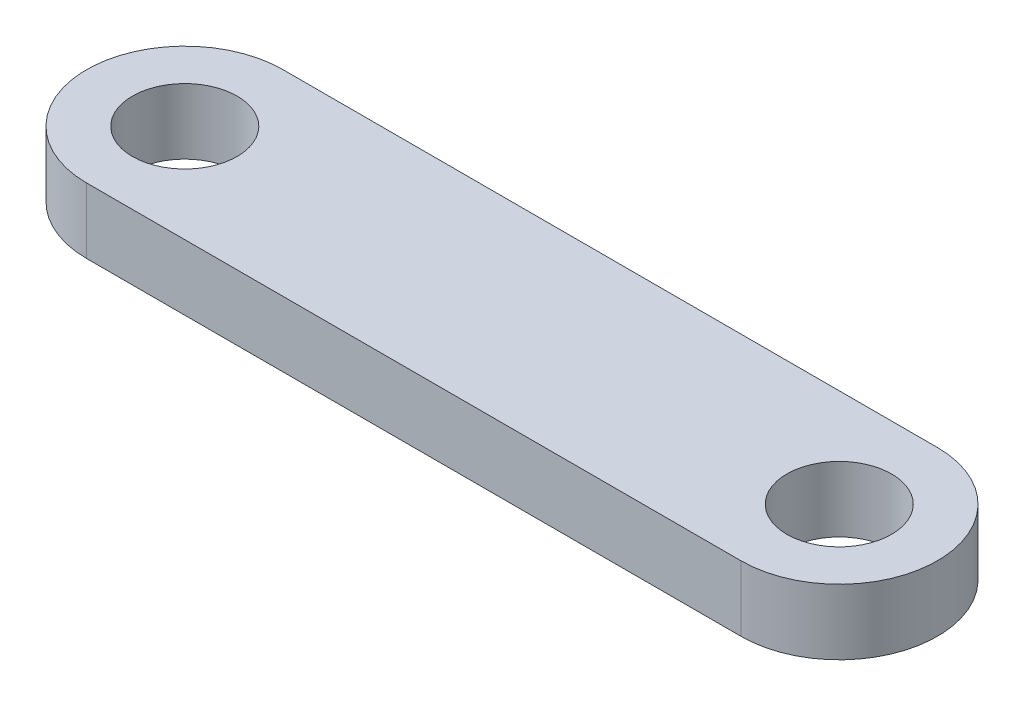
ISO-10303-21;
HEADER;
FILE_DESCRIPTION(('STEP AP214'),'2;1');
FILE_NAME('part.step','',(''),(''),'','','');
FILE_SCHEMA(('AUTOMOTIVE_DESIGN { 1 0 10303 214 1 1 1 1 }'));
ENDSEC;
DATA;
#1=APPLICATION_CONTEXT('core data for automotive mechanical design processes');
#2=APPLICATION_PROTOCOL_DEFINITION('international standard','automotive_design',2000,#1);
#3=PRODUCT_CONTEXT('',#1,'mechanical');
#4=PRODUCT('Part','Part','',(#3));
#5=PRODUCT_RELATED_PRODUCT_CATEGORY('part','',(#4));
#6=PRODUCT_DEFINITION_FORMATION('','',#4);
#7=PRODUCT_DEFINITION_CONTEXT('part definition',#1,'design');
#8=PRODUCT_DEFINITION('design','',#6,#7);
#9=PRODUCT_DEFINITION_SHAPE('','',#8);
#10=(LENGTH_UNIT() NAMED_UNIT(*) SI_UNIT(.MILLI.,.METRE.));
#11=(NAMED_UNIT(*) PLANE_ANGLE_UNIT() SI_UNIT($,.RADIAN.));
#12=(NAMED_UNIT(*) SI_UNIT($,.STERADIAN.) SOLID_ANGLE_UNIT());
#13=UNCERTAINTY_MEASURE_WITH_UNIT(LENGTH_MEASURE(1.E-05),#10,'distance_accuracy_value','');
#14=(GEOMETRIC_REPRESENTATION_CONTEXT(3) GLOBAL_UNCERTAINTY_ASSIGNED_CONTEXT((#13)) GLOBAL_UNIT_ASSIGNED_CONTEXT((#10,
#11,#12)) REPRESENTATION_CONTEXT('',''));
#15=CARTESIAN_POINT('',(0.,0.,0.));
#16=DIRECTION('',(0.,0.,1.));
#17=DIRECTION('',(1.,0.,0.));
#18=AXIS2_PLACEMENT_3D('',#15,#16,#17);
#19=CARTESIAN_POINT('',(-25.,2.5,0.));
#20=DIRECTION('',(0.,-1.,0.));
#21=DIRECTION('',(0.,0.,-1.));
#22=AXIS2_PLACEMENT_3D('',#19,#20,#21);
#23=CYLINDRICAL_SURFACE('',#22,7.5);
#24=CARTESIAN_POINT('',(-25.,-2.5,0.));
#25=DIRECTION('',(0.,1.,0.));
#26=DIRECTION('',(0.,0.,1.));
#27=AXIS2_PLACEMENT_3D('',#24,#25,#26);
#28=CIRCLE('',#27,7.5);
#29=CARTESIAN_POINT('',(-25.,-2.5,-7.5));
#30=VERTEX_POINT('',#29);
#31=CARTESIAN_POINT('',(-25.,-2.5,7.5));
#32=VERTEX_POINT('',#31);
#33=EDGE_CURVE('E102',#30,#32,#28,.T.);
#34=ORIENTED_EDGE('',*,*,#33,.T.);
#35=DIRECTION('',(0.,-1.,0.));
#36=VECTOR('',#35,1.);
#37=CARTESIAN_POINT('',(-25.,2.5,7.5));
#38=LINE('',#37,#36);
#39=CARTESIAN_POINT('',(-25.,2.5,7.5));
#40=VERTEX_POINT('',#39);
#41=EDGE_CURVE('E11',#40,#32,#38,.T.);
#42=ORIENTED_EDGE('',*,*,#41,.F.);
#43=CARTESIAN_POINT('',(-25.,2.5,0.));
#44=DIRECTION('',(0.,1.,0.));
#45=DIRECTION('',(0.,0.,1.));
#46=AXIS2_PLACEMENT_3D('',#43,#44,#45);
#47=CIRCLE('',#46,7.5);
#48=CARTESIAN_POINT('',(-25.,2.5,-7.5));
#49=VERTEX_POINT('',#48);
#50=EDGE_CURVE('E95',#49,#40,#47,.T.);
#51=ORIENTED_EDGE('',*,*,#50,.F.);
#52=DIRECTION('',(0.,-1.,0.));
#53=VECTOR('',#52,1.);
#54=CARTESIAN_POINT('',(-25.,2.5,-7.5));
#55=LINE('',#54,#53);
#56=EDGE_CURVE('E99',#49,#30,#55,.T.);
#57=ORIENTED_EDGE('',*,*,#56,.T.);
#58=EDGE_LOOP('',(#34,#42,#51,#57));
#59=FACE_BOUND('',#58,.T.);
#60=ADVANCED_FACE('F41',(#59),#23,.T.);
#61=CARTESIAN_POINT('',(-25.,2.5,7.5));
#62=DIRECTION('',(0.,0.,-1.));
#63=DIRECTION('',(-1.,0.,0.));
#64=AXIS2_PLACEMENT_3D('',#61,#62,#63);
#65=PLANE('',#64);
#66=DIRECTION('',(1.,0.,0.));
#67=VECTOR('',#66,1.);
#68=CARTESIAN_POINT('',(-25.,-2.5,7.5));
#69=LINE('',#68,#67);
#70=CARTESIAN_POINT('',(25.,-2.5,7.5));
#71=VERTEX_POINT('',#70);
#72=EDGE_CURVE('E96',#32,#71,#69,.T.);
#73=ORIENTED_EDGE('',*,*,#72,.T.);
#74=DIRECTION('',(0.,-1.,0.));
#75=VECTOR('',#74,1.);
#76=CARTESIAN_POINT('',(25.,2.5,7.5));
#77=LINE('',#76,#75);
#78=CARTESIAN_POINT('',(25.,2.5,7.5));
#79=VERTEX_POINT('',#78);
#80=EDGE_CURVE('E47',#79,#71,#77,.T.);
#81=ORIENTED_EDGE('',*,*,#80,.F.);
#82=DIRECTION('',(1.,0.,0.));
#83=VECTOR('',#82,1.);
#84=CARTESIAN_POINT('',(-25.,2.5,7.5));
#85=LINE('',#84,#83);
#86=EDGE_CURVE('E87',#40,#79,#85,.T.);
#87=ORIENTED_EDGE('',*,*,#86,.F.);
#88=ORIENTED_EDGE('',*,*,#41,.T.);
#89=EDGE_LOOP('',(#73,#81,#87,#88));
#90=FACE_BOUND('',#89,.T.);
#91=ADVANCED_FACE('F92',(#90),#65,.F.);
#92=CARTESIAN_POINT('',(25.,2.5,0.));
#93=DIRECTION('',(0.,-1.,0.));
#94=DIRECTION('',(0.,0.,-1.));
#95=AXIS2_PLACEMENT_3D('',#92,#93,#94);
#96=CYLINDRICAL_SURFACE('',#95,7.5);
#97=CARTESIAN_POINT('',(25.,-2.5,0.));
#98=DIRECTION('',(0.,1.,0.));
#99=DIRECTION('',(0.,0.,1.));
#100=AXIS2_PLACEMENT_3D('',#97,#98,#99);
#101=CIRCLE('',#100,7.5);
#102=CARTESIAN_POINT('',(25.,-2.5,-7.5));
#103=VERTEX_POINT('',#102);
#104=EDGE_CURVE('E74',#71,#103,#101,.T.);
#105=ORIENTED_EDGE('',*,*,#104,.T.);
#106=DIRECTION('',(0.,-1.,0.));
#107=VECTOR('',#106,1.);
#108=CARTESIAN_POINT('',(25.,2.5,-7.5));
#109=LINE('',#108,#107);
#110=CARTESIAN_POINT('',(25.,2.5,-7.5));
#111=VERTEX_POINT('',#110);
#112=EDGE_CURVE('E100',#111,#103,#109,.T.);
#113=ORIENTED_EDGE('',*,*,#112,.F.);
#114=CARTESIAN_POINT('',(25.,2.5,0.));
#115=DIRECTION('',(0.,1.,0.));
#116=DIRECTION('',(0.,0.,1.));
#117=AXIS2_PLACEMENT_3D('',#114,#115,#116);
#118=CIRCLE('',#117,7.5);
#119=EDGE_CURVE('E89',#79,#111,#118,.T.);
#120=ORIENTED_EDGE('',*,*,#119,.F.);
#121=ORIENTED_EDGE('',*,*,#80,.T.);
#122=EDGE_LOOP('',(#105,#113,#120,#121));
#123=FACE_BOUND('',#122,.T.);
#124=ADVANCED_FACE('F98',(#123),#96,.T.);
#125=CARTESIAN_POINT('',(-25.,2.5,-7.5));
#126=DIRECTION('',(0.,0.,1.));
#127=DIRECTION('',(1.,0.,0.));
#128=AXIS2_PLACEMENT_3D('',#125,#126,#127);
#129=PLANE('',#128);
#130=DIRECTION('',(-1.,0.,0.));
#131=VECTOR('',#130,1.);
#132=CARTESIAN_POINT('',(-25.,-2.5,-7.5));
#133=LINE('',#132,#131);
#134=EDGE_CURVE('E77',#103,#30,#133,.T.);
#135=ORIENTED_EDGE('',*,*,#134,.T.);
#136=ORIENTED_EDGE('',*,*,#56,.F.);
#137=DIRECTION('',(-1.,0.,0.));
#138=VECTOR('',#137,1.);
#139=CARTESIAN_POINT('',(-25.,2.5,-7.5));
#140=LINE('',#139,#138);
#141=EDGE_CURVE('E60',#111,#49,#140,.T.);
#142=ORIENTED_EDGE('',*,*,#141,.F.);
#143=ORIENTED_EDGE('',*,*,#112,.T.);
#144=EDGE_LOOP('',(#135,#136,#142,#143));
#145=FACE_BOUND('',#144,.T.);
#146=ADVANCED_FACE('F115',(#145),#129,.F.);
#147=CARTESIAN_POINT('',(-25.,2.5,0.));
#148=DIRECTION('',(0.,1.,0.));
#149=DIRECTION('',(0.,0.,1.));
#150=AXIS2_PLACEMENT_3D('',#147,#148,#149);
#151=PLANE('',#150);
#152=CARTESIAN_POINT('',(-25.,2.5,0.));
#153=DIRECTION('',(0.,1.,0.));
#154=DIRECTION('',(0.,0.,1.));
#155=AXIS2_PLACEMENT_3D('',#152,#153,#154);
#156=CIRCLE('',#155,4.);
#157=CARTESIAN_POINT('',(-25.,2.5,4.));
#158=VERTEX_POINT('',#157);
#159=EDGE_CURVE('E123',#158,#158,#156,.T.);
#160=ORIENTED_EDGE('',*,*,#159,.F.);
#161=EDGE_LOOP('',(#160));
#162=FACE_BOUND('',#161,.T.);
#163=CARTESIAN_POINT('',(25.,2.5,0.));
#164=DIRECTION('',(0.,1.,0.));
#165=DIRECTION('',(0.,0.,1.));
#166=AXIS2_PLACEMENT_3D('',#163,#164,#165);
#167=CIRCLE('',#166,4.);
#168=CARTESIAN_POINT('',(25.,2.5,4.));
#169=VERTEX_POINT('',#168);
#170=EDGE_CURVE('E124',#169,#169,#167,.T.);
#171=ORIENTED_EDGE('',*,*,#170,.F.);
#172=EDGE_LOOP('',(#171));
#173=FACE_BOUND('',#172,.T.);
#174=ORIENTED_EDGE('',*,*,#50,.T.);
#175=ORIENTED_EDGE('',*,*,#86,.T.);
#176=ORIENTED_EDGE('',*,*,#119,.T.);
#177=ORIENTED_EDGE('',*,*,#141,.T.);
#178=EDGE_LOOP('',(#174,#175,#176,#177));
#179=FACE_BOUND('',#178,.T.);
#180=ADVANCED_FACE('F86',(#162,#173,#179),#151,.T.);
#181=CARTESIAN_POINT('',(-25.,-2.5,0.));
#182=DIRECTION('',(0.,1.,0.));
#183=DIRECTION('',(0.,0.,1.));
#184=AXIS2_PLACEMENT_3D('',#181,#182,#183);
#185=PLANE('',#184);
#186=CARTESIAN_POINT('',(-25.,-2.5,0.));
#187=DIRECTION('',(0.,1.,0.));
#188=DIRECTION('',(0.,0.,1.));
#189=AXIS2_PLACEMENT_3D('',#186,#187,#188);
#190=CIRCLE('',#189,4.);
#191=CARTESIAN_POINT('',(-25.,-2.5,4.));
#192=VERTEX_POINT('',#191);
#193=EDGE_CURVE('E110',#192,#192,#190,.T.);
#194=ORIENTED_EDGE('',*,*,#193,.T.);
#195=EDGE_LOOP('',(#194));
#196=FACE_BOUND('',#195,.T.);
#197=CARTESIAN_POINT('',(25.,-2.5,0.));
#198=DIRECTION('',(0.,1.,0.));
#199=DIRECTION('',(0.,0.,1.));
#200=AXIS2_PLACEMENT_3D('',#197,#198,#199);
#201=CIRCLE('',#200,4.);
#202=CARTESIAN_POINT('',(25.,-2.5,4.));
#203=VERTEX_POINT('',#202);
#204=EDGE_CURVE('E120',#203,#203,#201,.T.);
#205=ORIENTED_EDGE('',*,*,#204,.T.);
#206=EDGE_LOOP('',(#205));
#207=FACE_BOUND('',#206,.T.);
#208=ORIENTED_EDGE('',*,*,#33,.F.);
#209=ORIENTED_EDGE('',*,*,#134,.F.);
#210=ORIENTED_EDGE('',*,*,#104,.F.);
#211=ORIENTED_EDGE('',*,*,#72,.F.);
#212=EDGE_LOOP('',(#208,#209,#210,#211));
#213=FACE_BOUND('',#212,.T.);
#214=ADVANCED_FACE('F113',(#196,#207,#213),#185,.F.);
#215=CARTESIAN_POINT('',(25.,-2.5,0.));
#216=DIRECTION('',(0.,1.,0.));
#217=DIRECTION('',(0.,0.,1.));
#218=AXIS2_PLACEMENT_3D('',#215,#216,#217);
#219=CYLINDRICAL_SURFACE('',#218,4.);
#220=ORIENTED_EDGE('',*,*,#204,.F.);
#221=EDGE_LOOP('',(#220));
#222=FACE_BOUND('',#221,.T.);
#223=ORIENTED_EDGE('',*,*,#170,.T.);
#224=EDGE_LOOP('',(#223));
#225=FACE_BOUND('',#224,.T.);
#226=ADVANCED_FACE('F132',(#222,#225),#219,.F.);
#227=CARTESIAN_POINT('',(-25.,-2.5,0.));
#228=DIRECTION('',(0.,1.,0.));
#229=DIRECTION('',(0.,0.,1.));
#230=AXIS2_PLACEMENT_3D('',#227,#228,#229);
#231=CYLINDRICAL_SURFACE('',#230,4.);
#232=ORIENTED_EDGE('',*,*,#193,.F.);
#233=EDGE_LOOP('',(#232));
#234=FACE_BOUND('',#233,.T.);
#235=ORIENTED_EDGE('',*,*,#159,.T.);
#236=EDGE_LOOP('',(#235));
#237=FACE_BOUND('',#236,.T.);
#238=ADVANCED_FACE('F131',(#234,#237),#231,.F.);
#239=CLOSED_SHELL('',(#60,#91,#124,#146,#180,#214,#226,#238));
#240=MANIFOLD_SOLID_BREP('B2',#239);
#241=ADVANCED_BREP_SHAPE_REPRESENTATION('',(#18,#240),#14);
#242=SHAPE_DEFINITION_REPRESENTATION(#9,#241);
ENDSEC;
END-ISO-10303-21;
